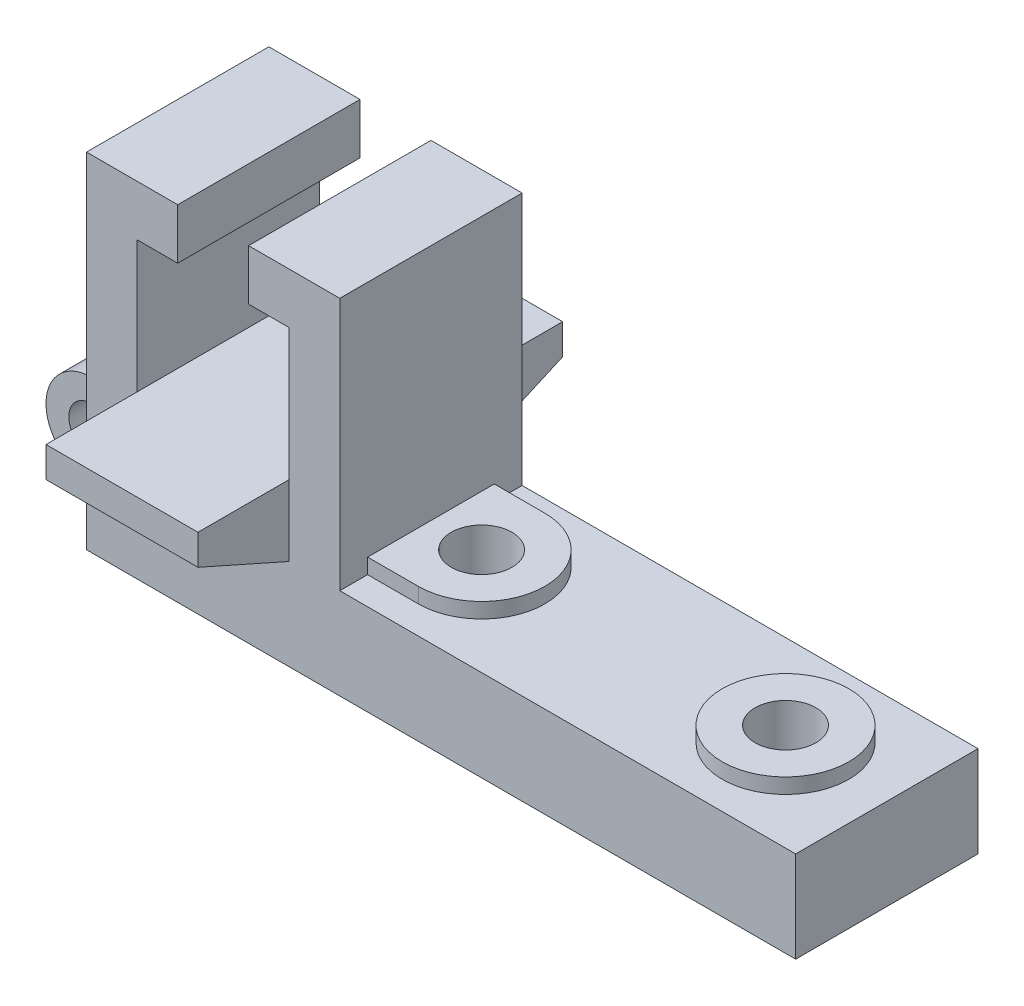
ISO-10303-21;
HEADER;
FILE_DESCRIPTION(('STEP AP214'),'2;1');
FILE_NAME('part.step','',(''),(''),'','','');
FILE_SCHEMA(('AUTOMOTIVE_DESIGN { 1 0 10303 214 1 1 1 1 }'));
ENDSEC;
DATA;
#1=APPLICATION_CONTEXT('core data for automotive mechanical design processes');
#2=APPLICATION_PROTOCOL_DEFINITION('international standard','automotive_design',2000,#1);
#3=PRODUCT_CONTEXT('',#1,'mechanical');
#4=PRODUCT('Part','Part','',(#3));
#5=PRODUCT_RELATED_PRODUCT_CATEGORY('part','',(#4));
#6=PRODUCT_DEFINITION_FORMATION('','',#4);
#7=PRODUCT_DEFINITION_CONTEXT('part definition',#1,'design');
#8=PRODUCT_DEFINITION('design','',#6,#7);
#9=PRODUCT_DEFINITION_SHAPE('','',#8);
#10=(LENGTH_UNIT() NAMED_UNIT(*) SI_UNIT(.MILLI.,.METRE.));
#11=(NAMED_UNIT(*) PLANE_ANGLE_UNIT() SI_UNIT($,.RADIAN.));
#12=(NAMED_UNIT(*) SI_UNIT($,.STERADIAN.) SOLID_ANGLE_UNIT());
#13=UNCERTAINTY_MEASURE_WITH_UNIT(LENGTH_MEASURE(1.E-05),#10,'distance_accuracy_value','');
#14=(GEOMETRIC_REPRESENTATION_CONTEXT(3) GLOBAL_UNCERTAINTY_ASSIGNED_CONTEXT((#13)) GLOBAL_UNIT_ASSIGNED_CONTEXT((#10,
#11,#12)) REPRESENTATION_CONTEXT('',''));
#15=CARTESIAN_POINT('',(0.,0.,0.));
#16=DIRECTION('',(0.,0.,1.));
#17=DIRECTION('',(1.,0.,0.));
#18=AXIS2_PLACEMENT_3D('',#15,#16,#17);
#19=CARTESIAN_POINT('',(140.,18.,36.));
#20=DIRECTION('',(0.,-1.,0.));
#21=DIRECTION('',(0.,0.,-1.));
#22=AXIS2_PLACEMENT_3D('',#19,#20,#21);
#23=PLANE('',#22);
#24=CARTESIAN_POINT('',(120.,18.,18.));
#25=DIRECTION('',(0.,-1.,0.));
#26=DIRECTION('',(0.,0.,-1.));
#27=AXIS2_PLACEMENT_3D('',#24,#25,#26);
#28=CIRCLE('',#27,12.5);
#29=CARTESIAN_POINT('',(120.,18.,5.50000000000001));
#30=VERTEX_POINT('',#29);
#31=EDGE_CURVE('E11',#30,#30,#28,.F.);
#32=ORIENTED_EDGE('',*,*,#31,.F.);
#33=EDGE_LOOP('',(#32));
#34=FACE_BOUND('',#33,.T.);
#35=DIRECTION('',(-1.,0.,0.));
#36=VECTOR('',#35,1.);
#37=CARTESIAN_POINT('',(60.,18.,5.49999999999999));
#38=LINE('',#37,#36);
#39=CARTESIAN_POINT('',(60.,18.,5.49999999999999));
#40=VERTEX_POINT('',#39);
#41=CARTESIAN_POINT('',(50.,18.,5.5));
#42=VERTEX_POINT('',#41);
#43=EDGE_CURVE('E58',#40,#42,#38,.T.);
#44=ORIENTED_EDGE('',*,*,#43,.F.);
#45=CARTESIAN_POINT('',(60.,18.,18.));
#46=DIRECTION('',(0.,1.,0.));
#47=DIRECTION('',(0.,0.,1.));
#48=AXIS2_PLACEMENT_3D('',#45,#46,#47);
#49=CIRCLE('',#48,12.5);
#50=CARTESIAN_POINT('',(60.,18.,30.5));
#51=VERTEX_POINT('',#50);
#52=EDGE_CURVE('E64',#51,#40,#49,.T.);
#53=ORIENTED_EDGE('',*,*,#52,.F.);
#54=DIRECTION('',(1.,0.,0.));
#55=VECTOR('',#54,1.);
#56=CARTESIAN_POINT('',(50.,18.,30.5));
#57=LINE('',#56,#55);
#58=CARTESIAN_POINT('',(50.,18.,30.5));
#59=VERTEX_POINT('',#58);
#60=EDGE_CURVE('E247',#59,#51,#57,.T.);
#61=ORIENTED_EDGE('',*,*,#60,.F.);
#62=DIRECTION('',(0.,0.,-1.));
#63=VECTOR('',#62,1.);
#64=CARTESIAN_POINT('',(50.,18.,36.));
#65=LINE('',#64,#63);
#66=CARTESIAN_POINT('',(50.,18.,36.));
#67=VERTEX_POINT('',#66);
#68=EDGE_CURVE('E323',#67,#59,#65,.T.);
#69=ORIENTED_EDGE('',*,*,#68,.F.);
#70=DIRECTION('',(-1.,0.,0.));
#71=VECTOR('',#70,1.);
#72=CARTESIAN_POINT('',(140.,18.,36.));
#73=LINE('',#72,#71);
#74=CARTESIAN_POINT('',(140.,18.,36.));
#75=VERTEX_POINT('',#74);
#76=EDGE_CURVE('E421',#75,#67,#73,.T.);
#77=ORIENTED_EDGE('',*,*,#76,.F.);
#78=DIRECTION('',(0.,0.,-1.));
#79=VECTOR('',#78,1.);
#80=CARTESIAN_POINT('',(140.,18.,36.));
#81=LINE('',#80,#79);
#82=CARTESIAN_POINT('',(140.,18.,0.));
#83=VERTEX_POINT('',#82);
#84=EDGE_CURVE('E428',#75,#83,#81,.T.);
#85=ORIENTED_EDGE('',*,*,#84,.T.);
#86=DIRECTION('',(-1.,0.,0.));
#87=VECTOR('',#86,1.);
#88=CARTESIAN_POINT('',(140.,18.,0.));
#89=LINE('',#88,#87);
#90=CARTESIAN_POINT('',(50.,18.,0.));
#91=VERTEX_POINT('',#90);
#92=EDGE_CURVE('E418',#83,#91,#89,.T.);
#93=ORIENTED_EDGE('',*,*,#92,.T.);
#94=EDGE_CURVE('E328',#42,#91,#65,.T.);
#95=ORIENTED_EDGE('',*,*,#94,.F.);
#96=EDGE_LOOP('',(#44,#53,#61,#69,#77,#85,#93,#95));
#97=FACE_BOUND('',#96,.T.);
#98=ADVANCED_FACE('F44',(#34,#97),#23,.F.);
#99=CARTESIAN_POINT('',(50.,18.,36.));
#100=DIRECTION('',(1.,0.,0.));
#101=DIRECTION('',(0.,0.,-1.));
#102=AXIS2_PLACEMENT_3D('',#99,#100,#101);
#103=PLANE('',#102);
#104=DIRECTION('',(0.,0.,1.));
#105=VECTOR('',#104,1.);
#106=CARTESIAN_POINT('',(50.,21.,5.49999999999999));
#107=LINE('',#106,#105);
#108=CARTESIAN_POINT('',(50.,21.,5.5));
#109=VERTEX_POINT('',#108);
#110=CARTESIAN_POINT('',(50.,21.,30.5));
#111=VERTEX_POINT('',#110);
#112=EDGE_CURVE('E238',#109,#111,#107,.T.);
#113=ORIENTED_EDGE('',*,*,#112,.F.);
#114=DIRECTION('',(0.,-1.,0.));
#115=VECTOR('',#114,1.);
#116=CARTESIAN_POINT('',(50.,21.,5.49999999999999));
#117=LINE('',#116,#115);
#118=EDGE_CURVE('E232',#109,#42,#117,.T.);
#119=ORIENTED_EDGE('',*,*,#118,.T.);
#120=ORIENTED_EDGE('',*,*,#94,.T.);
#121=DIRECTION('',(0.,-1.,0.));
#122=VECTOR('',#121,1.);
#123=CARTESIAN_POINT('',(50.,18.,0.));
#124=LINE('',#123,#122);
#125=CARTESIAN_POINT('',(50.,68.,0.));
#126=VERTEX_POINT('',#125);
#127=EDGE_CURVE('E321',#126,#91,#124,.T.);
#128=ORIENTED_EDGE('',*,*,#127,.F.);
#129=DIRECTION('',(0.,0.,-1.));
#130=VECTOR('',#129,1.);
#131=CARTESIAN_POINT('',(50.,68.,36.));
#132=LINE('',#131,#130);
#133=CARTESIAN_POINT('',(50.,68.,36.));
#134=VERTEX_POINT('',#133);
#135=EDGE_CURVE('E327',#134,#126,#132,.T.);
#136=ORIENTED_EDGE('',*,*,#135,.F.);
#137=DIRECTION('',(0.,-1.,0.));
#138=VECTOR('',#137,1.);
#139=CARTESIAN_POINT('',(50.,18.,36.));
#140=LINE('',#139,#138);
#141=EDGE_CURVE('E304',#134,#67,#140,.T.);
#142=ORIENTED_EDGE('',*,*,#141,.T.);
#143=ORIENTED_EDGE('',*,*,#68,.T.);
#144=DIRECTION('',(0.,-1.,0.));
#145=VECTOR('',#144,1.);
#146=CARTESIAN_POINT('',(50.,21.,30.5));
#147=LINE('',#146,#145);
#148=EDGE_CURVE('E256',#111,#59,#147,.T.);
#149=ORIENTED_EDGE('',*,*,#148,.F.);
#150=EDGE_LOOP('',(#113,#119,#120,#128,#136,#142,#143,#149));
#151=FACE_BOUND('',#150,.T.);
#152=ADVANCED_FACE('F523',(#151),#103,.T.);
#153=CARTESIAN_POINT('',(0.,18.,30.));
#154=DIRECTION('',(0.,1.,0.));
#155=DIRECTION('',(0.,0.,1.));
#156=AXIS2_PLACEMENT_3D('',#153,#154,#155);
#157=PLANE('',#156);
#158=DIRECTION('',(0.,0.,-1.));
#159=VECTOR('',#158,1.);
#160=CARTESIAN_POINT('',(-11.,18.,30.));
#161=LINE('',#160,#159);
#162=CARTESIAN_POINT('',(-11.,18.,24.));
#163=VERTEX_POINT('',#162);
#164=CARTESIAN_POINT('',(-11.,18.,12.));
#165=VERTEX_POINT('',#164);
#166=EDGE_CURVE('E287',#163,#165,#161,.T.);
#167=ORIENTED_EDGE('',*,*,#166,.F.);
#168=DIRECTION('',(-1.,0.,0.));
#169=VECTOR('',#168,1.);
#170=CARTESIAN_POINT('',(0.,18.,24.));
#171=LINE('',#170,#169);
#172=CARTESIAN_POINT('',(0.,18.,24.));
#173=VERTEX_POINT('',#172);
#174=EDGE_CURVE('E262',#173,#163,#171,.T.);
#175=ORIENTED_EDGE('',*,*,#174,.F.);
#176=DIRECTION('',(0.,0.,-1.));
#177=VECTOR('',#176,1.);
#178=CARTESIAN_POINT('',(0.,18.,30.));
#179=LINE('',#178,#177);
#180=CARTESIAN_POINT('',(0.,18.,12.));
#181=VERTEX_POINT('',#180);
#182=EDGE_CURVE('E286',#173,#181,#179,.T.);
#183=ORIENTED_EDGE('',*,*,#182,.T.);
#184=DIRECTION('',(1.,0.,0.));
#185=VECTOR('',#184,1.);
#186=CARTESIAN_POINT('',(0.,18.,12.));
#187=LINE('',#186,#185);
#188=EDGE_CURVE('E279',#165,#181,#187,.T.);
#189=ORIENTED_EDGE('',*,*,#188,.F.);
#190=EDGE_LOOP('',(#167,#175,#183,#189));
#191=FACE_BOUND('',#190,.T.);
#192=ADVANCED_FACE('F532',(#191),#157,.T.);
#193=CARTESIAN_POINT('',(-11.,9.,30.));
#194=DIRECTION('',(0.,0.,-1.));
#195=DIRECTION('',(-1.,0.,0.));
#196=AXIS2_PLACEMENT_3D('',#193,#194,#195);
#197=CYLINDRICAL_SURFACE('',#196,9.);
#198=DIRECTION('',(0.,0.,-1.));
#199=VECTOR('',#198,1.);
#200=CARTESIAN_POINT('',(-11.,0.,30.));
#201=LINE('',#200,#199);
#202=CARTESIAN_POINT('',(-10.9999999999999,0.,24.));
#203=VERTEX_POINT('',#202);
#204=CARTESIAN_POINT('',(-11.,0.,12.));
#205=VERTEX_POINT('',#204);
#206=EDGE_CURVE('E289',#203,#205,#201,.T.);
#207=ORIENTED_EDGE('',*,*,#206,.F.);
#208=CARTESIAN_POINT('',(-11.,9.,24.));
#209=DIRECTION('',(0.,0.,1.));
#210=DIRECTION('',(1.,0.,0.));
#211=AXIS2_PLACEMENT_3D('',#208,#209,#210);
#212=CIRCLE('',#211,9.);
#213=EDGE_CURVE('E269',#163,#203,#212,.T.);
#214=ORIENTED_EDGE('',*,*,#213,.F.);
#215=ORIENTED_EDGE('',*,*,#166,.T.);
#216=CARTESIAN_POINT('',(-11.,9.,12.));
#217=DIRECTION('',(0.,0.,-1.));
#218=DIRECTION('',(-1.,0.,0.));
#219=AXIS2_PLACEMENT_3D('',#216,#217,#218);
#220=CIRCLE('',#219,9.);
#221=EDGE_CURVE('E280',#205,#165,#220,.T.);
#222=ORIENTED_EDGE('',*,*,#221,.F.);
#223=EDGE_LOOP('',(#207,#214,#215,#222));
#224=FACE_BOUND('',#223,.T.);
#225=ADVANCED_FACE('F571',(#224),#197,.T.);
#226=CARTESIAN_POINT('',(0.,18.,36.));
#227=DIRECTION('',(1.,0.,0.));
#228=DIRECTION('',(0.,0.,-1.));
#229=AXIS2_PLACEMENT_3D('',#226,#227,#228);
#230=PLANE('',#229);
#231=ORIENTED_EDGE('',*,*,#182,.F.);
#232=DIRECTION('',(0.,1.,0.));
#233=VECTOR('',#232,1.);
#234=CARTESIAN_POINT('',(0.,0.,24.));
#235=LINE('',#234,#233);
#236=CARTESIAN_POINT('',(0.,0.,24.));
#237=VERTEX_POINT('',#236);
#238=EDGE_CURVE('E261',#237,#173,#235,.T.);
#239=ORIENTED_EDGE('',*,*,#238,.F.);
#240=DIRECTION('',(0.,0.,-1.));
#241=VECTOR('',#240,1.);
#242=CARTESIAN_POINT('',(0.,0.,36.));
#243=LINE('',#242,#241);
#244=CARTESIAN_POINT('',(0.,0.,36.));
#245=VERTEX_POINT('',#244);
#246=EDGE_CURVE('E437',#245,#237,#243,.T.);
#247=ORIENTED_EDGE('',*,*,#246,.F.);
#248=DIRECTION('',(0.,-1.,0.));
#249=VECTOR('',#248,1.);
#250=CARTESIAN_POINT('',(0.,18.,36.));
#251=LINE('',#250,#249);
#252=CARTESIAN_POINT('',(0.,68.,36.));
#253=VERTEX_POINT('',#252);
#254=EDGE_CURVE('E414',#253,#245,#251,.T.);
#255=ORIENTED_EDGE('',*,*,#254,.F.);
#256=DIRECTION('',(0.,0.,1.));
#257=VECTOR('',#256,1.);
#258=CARTESIAN_POINT('',(0.,68.,0.));
#259=LINE('',#258,#257);
#260=CARTESIAN_POINT('',(0.,68.,0.));
#261=VERTEX_POINT('',#260);
#262=EDGE_CURVE('E403',#261,#253,#259,.T.);
#263=ORIENTED_EDGE('',*,*,#262,.F.);
#264=DIRECTION('',(0.,-1.,0.));
#265=VECTOR('',#264,1.);
#266=CARTESIAN_POINT('',(0.,18.,0.));
#267=LINE('',#266,#265);
#268=CARTESIAN_POINT('',(0.,0.,0.));
#269=VERTEX_POINT('',#268);
#270=EDGE_CURVE('E407',#261,#269,#267,.T.);
#271=ORIENTED_EDGE('',*,*,#270,.T.);
#272=DIRECTION('',(0.,0.,-1.));
#273=VECTOR('',#272,1.);
#274=CARTESIAN_POINT('',(0.,0.,12.));
#275=LINE('',#274,#273);
#276=CARTESIAN_POINT('',(0.,0.,12.));
#277=VERTEX_POINT('',#276);
#278=EDGE_CURVE('E283',#277,#269,#275,.T.);
#279=ORIENTED_EDGE('',*,*,#278,.F.);
#280=DIRECTION('',(0.,-1.,0.));
#281=VECTOR('',#280,1.);
#282=CARTESIAN_POINT('',(0.,0.,12.));
#283=LINE('',#282,#281);
#284=EDGE_CURVE('E272',#181,#277,#283,.T.);
#285=ORIENTED_EDGE('',*,*,#284,.F.);
#286=EDGE_LOOP('',(#231,#239,#247,#255,#263,#271,#279,#285));
#287=FACE_BOUND('',#286,.T.);
#288=ADVANCED_FACE('F50',(#287),#230,.F.);
#289=CARTESIAN_POINT('',(40.,0.,0.));
#290=DIRECTION('',(-1.,0.,0.));
#291=DIRECTION('',(0.,0.,1.));
#292=AXIS2_PLACEMENT_3D('',#289,#290,#291);
#293=PLANE('',#292);
#294=DIRECTION('',(0.,1.,0.));
#295=VECTOR('',#294,1.);
#296=CARTESIAN_POINT('',(40.,18.,0.));
#297=LINE('',#296,#295);
#298=CARTESIAN_POINT('',(40.,18.,0.));
#299=VERTEX_POINT('',#298);
#300=CARTESIAN_POINT('',(40.,32.,0.));
#301=VERTEX_POINT('',#300);
#302=EDGE_CURVE('E307',#299,#301,#297,.T.);
#303=ORIENTED_EDGE('',*,*,#302,.F.);
#304=DIRECTION('',(0.,0.406138466053448,-0.913811548620257));
#305=VECTOR('',#304,1.);
#306=CARTESIAN_POINT('',(40.,26.,-18.));
#307=LINE('',#306,#305);
#308=CARTESIAN_POINT('',(40.,26.,-18.));
#309=VERTEX_POINT('',#308);
#310=EDGE_CURVE('E340',#299,#309,#307,.T.);
#311=ORIENTED_EDGE('',*,*,#310,.T.);
#312=DIRECTION('',(0.,1.,0.));
#313=VECTOR('',#312,1.);
#314=CARTESIAN_POINT('',(40.,32.,-18.));
#315=LINE('',#314,#313);
#316=CARTESIAN_POINT('',(40.,32.,-18.));
#317=VERTEX_POINT('',#316);
#318=EDGE_CURVE('E339',#309,#317,#315,.T.);
#319=ORIENTED_EDGE('',*,*,#318,.T.);
#320=DIRECTION('',(0.,0.,1.));
#321=VECTOR('',#320,1.);
#322=CARTESIAN_POINT('',(40.,32.,18.));
#323=LINE('',#322,#321);
#324=EDGE_CURVE('E342',#317,#301,#323,.T.);
#325=ORIENTED_EDGE('',*,*,#324,.T.);
#326=EDGE_LOOP('',(#303,#311,#319,#325));
#327=FACE_BOUND('',#326,.T.);
#328=ADVANCED_FACE('F496',(#327),#293,.F.);
#329=CARTESIAN_POINT('',(10.,18.,0.));
#330=DIRECTION('',(1.,0.,0.));
#331=DIRECTION('',(0.,0.,-1.));
#332=AXIS2_PLACEMENT_3D('',#329,#330,#331);
#333=PLANE('',#332);
#334=DIRECTION('',(0.,1.,0.));
#335=VECTOR('',#334,1.);
#336=CARTESIAN_POINT('',(10.,18.,36.));
#337=LINE('',#336,#335);
#338=CARTESIAN_POINT('',(10.,32.,36.));
#339=VERTEX_POINT('',#338);
#340=CARTESIAN_POINT('',(10.,58.,36.));
#341=VERTEX_POINT('',#340);
#342=EDGE_CURVE('E377',#339,#341,#337,.T.);
#343=ORIENTED_EDGE('',*,*,#342,.F.);
#344=DIRECTION('',(0.,0.,-1.));
#345=VECTOR('',#344,1.);
#346=CARTESIAN_POINT('',(10.,32.,0.));
#347=LINE('',#346,#345);
#348=CARTESIAN_POINT('',(10.,32.,0.));
#349=VERTEX_POINT('',#348);
#350=EDGE_CURVE('E52',#339,#349,#347,.T.);
#351=ORIENTED_EDGE('',*,*,#350,.T.);
#352=DIRECTION('',(0.,1.,0.));
#353=VECTOR('',#352,1.);
#354=CARTESIAN_POINT('',(10.,18.,0.));
#355=LINE('',#354,#353);
#356=CARTESIAN_POINT('',(10.,58.,0.));
#357=VERTEX_POINT('',#356);
#358=EDGE_CURVE('E384',#349,#357,#355,.T.);
#359=ORIENTED_EDGE('',*,*,#358,.T.);
#360=DIRECTION('',(0.,0.,1.));
#361=VECTOR('',#360,1.);
#362=CARTESIAN_POINT('',(10.,58.,0.));
#363=LINE('',#362,#361);
#364=EDGE_CURVE('E395',#357,#341,#363,.T.);
#365=ORIENTED_EDGE('',*,*,#364,.T.);
#366=EDGE_LOOP('',(#343,#351,#359,#365));
#367=FACE_BOUND('',#366,.T.);
#368=ADVANCED_FACE('F444',(#367),#333,.T.);
#369=CARTESIAN_POINT('',(0.,0.,36.));
#370=DIRECTION('',(0.,1.,0.));
#371=DIRECTION('',(0.,0.,1.));
#372=AXIS2_PLACEMENT_3D('',#369,#370,#371);
#373=PLANE('',#372);
#374=CARTESIAN_POINT('',(120.,0.,18.));
#375=DIRECTION('',(0.,1.,0.));
#376=DIRECTION('',(0.,0.,1.));
#377=AXIS2_PLACEMENT_3D('',#374,#375,#376);
#378=CIRCLE('',#377,6.);
#379=CARTESIAN_POINT('',(120.,0.,24.));
#380=VERTEX_POINT('',#379);
#381=EDGE_CURVE('E552',#380,#380,#378,.T.);
#382=ORIENTED_EDGE('',*,*,#381,.T.);
#383=EDGE_LOOP('',(#382));
#384=FACE_BOUND('',#383,.T.);
#385=CARTESIAN_POINT('',(60.,0.,18.));
#386=DIRECTION('',(0.,1.,0.));
#387=DIRECTION('',(0.,0.,1.));
#388=AXIS2_PLACEMENT_3D('',#385,#386,#387);
#389=CIRCLE('',#388,6.);
#390=CARTESIAN_POINT('',(60.,0.,24.));
#391=VERTEX_POINT('',#390);
#392=EDGE_CURVE('E558',#391,#391,#389,.T.);
#393=ORIENTED_EDGE('',*,*,#392,.T.);
#394=EDGE_LOOP('',(#393));
#395=FACE_BOUND('',#394,.T.);
#396=ORIENTED_EDGE('',*,*,#246,.T.);
#397=DIRECTION('',(1.,0.,0.));
#398=VECTOR('',#397,1.);
#399=CARTESIAN_POINT('',(-10.9999999999999,0.,24.));
#400=LINE('',#399,#398);
#401=EDGE_CURVE('E270',#203,#237,#400,.T.);
#402=ORIENTED_EDGE('',*,*,#401,.F.);
#403=ORIENTED_EDGE('',*,*,#206,.T.);
#404=DIRECTION('',(-1.,0.,0.));
#405=VECTOR('',#404,1.);
#406=CARTESIAN_POINT('',(-11.,0.,12.));
#407=LINE('',#406,#405);
#408=EDGE_CURVE('E274',#277,#205,#407,.T.);
#409=ORIENTED_EDGE('',*,*,#408,.F.);
#410=ORIENTED_EDGE('',*,*,#278,.T.);
#411=DIRECTION('',(1.,0.,0.));
#412=VECTOR('',#411,1.);
#413=CARTESIAN_POINT('',(0.,0.,0.));
#414=LINE('',#413,#412);
#415=CARTESIAN_POINT('',(140.,0.,0.));
#416=VERTEX_POINT('',#415);
#417=EDGE_CURVE('E426',#269,#416,#414,.T.);
#418=ORIENTED_EDGE('',*,*,#417,.T.);
#419=DIRECTION('',(0.,0.,-1.));
#420=VECTOR('',#419,1.);
#421=CARTESIAN_POINT('',(140.,0.,36.));
#422=LINE('',#421,#420);
#423=CARTESIAN_POINT('',(140.,0.,36.));
#424=VERTEX_POINT('',#423);
#425=EDGE_CURVE('E436',#424,#416,#422,.T.);
#426=ORIENTED_EDGE('',*,*,#425,.F.);
#427=DIRECTION('',(1.,0.,0.));
#428=VECTOR('',#427,1.);
#429=CARTESIAN_POINT('',(0.,0.,36.));
#430=LINE('',#429,#428);
#431=EDGE_CURVE('E420',#245,#424,#430,.T.);
#432=ORIENTED_EDGE('',*,*,#431,.F.);
#433=EDGE_LOOP('',(#396,#402,#403,#409,#410,#418,#426,#432));
#434=FACE_BOUND('',#433,.T.);
#435=ADVANCED_FACE('F539',(#384,#395,#434),#373,.F.);
#436=CARTESIAN_POINT('',(140.,0.,36.));
#437=DIRECTION('',(-1.,0.,0.));
#438=DIRECTION('',(0.,0.,1.));
#439=AXIS2_PLACEMENT_3D('',#436,#437,#438);
#440=PLANE('',#439);
#441=DIRECTION('',(0.,1.,0.));
#442=VECTOR('',#441,1.);
#443=CARTESIAN_POINT('',(140.,0.,0.));
#444=LINE('',#443,#442);
#445=EDGE_CURVE('E427',#416,#83,#444,.T.);
#446=ORIENTED_EDGE('',*,*,#445,.T.);
#447=ORIENTED_EDGE('',*,*,#84,.F.);
#448=DIRECTION('',(0.,1.,0.));
#449=VECTOR('',#448,1.);
#450=CARTESIAN_POINT('',(140.,0.,36.));
#451=LINE('',#450,#449);
#452=EDGE_CURVE('E423',#424,#75,#451,.T.);
#453=ORIENTED_EDGE('',*,*,#452,.F.);
#454=ORIENTED_EDGE('',*,*,#425,.T.);
#455=EDGE_LOOP('',(#446,#447,#453,#454));
#456=FACE_BOUND('',#455,.T.);
#457=ADVANCED_FACE('F537',(#456),#440,.F.);
#458=CARTESIAN_POINT('',(0.,0.,36.));
#459=DIRECTION('',(0.,0.,1.));
#460=DIRECTION('',(1.,0.,0.));
#461=AXIS2_PLACEMENT_3D('',#458,#459,#460);
#462=PLANE('',#461);
#463=ORIENTED_EDGE('',*,*,#254,.T.);
#464=ORIENTED_EDGE('',*,*,#431,.T.);
#465=ORIENTED_EDGE('',*,*,#452,.T.);
#466=ORIENTED_EDGE('',*,*,#76,.T.);
#467=ORIENTED_EDGE('',*,*,#141,.F.);
#468=DIRECTION('',(1.,0.,0.));
#469=VECTOR('',#468,1.);
#470=CARTESIAN_POINT('',(50.,68.,36.));
#471=LINE('',#470,#469);
#472=CARTESIAN_POINT('',(32.,68.,36.));
#473=VERTEX_POINT('',#472);
#474=EDGE_CURVE('E305',#473,#134,#471,.T.);
#475=ORIENTED_EDGE('',*,*,#474,.F.);
#476=DIRECTION('',(0.,1.,0.));
#477=VECTOR('',#476,1.);
#478=CARTESIAN_POINT('',(32.,68.,36.));
#479=LINE('',#478,#477);
#480=CARTESIAN_POINT('',(32.,58.,36.));
#481=VERTEX_POINT('',#480);
#482=EDGE_CURVE('E299',#481,#473,#479,.T.);
#483=ORIENTED_EDGE('',*,*,#482,.F.);
#484=DIRECTION('',(-1.,0.,0.));
#485=VECTOR('',#484,1.);
#486=CARTESIAN_POINT('',(40.,58.,36.));
#487=LINE('',#486,#485);
#488=CARTESIAN_POINT('',(40.,58.,36.));
#489=VERTEX_POINT('',#488);
#490=EDGE_CURVE('E294',#489,#481,#487,.T.);
#491=ORIENTED_EDGE('',*,*,#490,.F.);
#492=DIRECTION('',(0.,1.,0.));
#493=VECTOR('',#492,1.);
#494=CARTESIAN_POINT('',(40.,18.,36.));
#495=LINE('',#494,#493);
#496=CARTESIAN_POINT('',(40.,32.,36.));
#497=VERTEX_POINT('',#496);
#498=EDGE_CURVE('E298',#497,#489,#495,.T.);
#499=ORIENTED_EDGE('',*,*,#498,.F.);
#500=CARTESIAN_POINT('',(40.,18.,36.));
#501=VERTEX_POINT('',#500);
#502=EDGE_CURVE('E291',#501,#497,#495,.T.);
#503=ORIENTED_EDGE('',*,*,#502,.F.);
#504=DIRECTION('',(-1.,0.,0.));
#505=VECTOR('',#504,1.);
#506=CARTESIAN_POINT('',(40.,18.,36.));
#507=LINE('',#506,#505);
#508=CARTESIAN_POINT('',(10.,18.,36.));
#509=VERTEX_POINT('',#508);
#510=EDGE_CURVE('E349',#501,#509,#507,.T.);
#511=ORIENTED_EDGE('',*,*,#510,.T.);
#512=EDGE_CURVE('E393',#509,#339,#337,.T.);
#513=ORIENTED_EDGE('',*,*,#512,.T.);
#514=ORIENTED_EDGE('',*,*,#342,.T.);
#515=DIRECTION('',(1.,0.,0.));
#516=VECTOR('',#515,1.);
#517=CARTESIAN_POINT('',(10.,58.,36.));
#518=LINE('',#517,#516);
#519=CARTESIAN_POINT('',(18.,58.,36.));
#520=VERTEX_POINT('',#519);
#521=EDGE_CURVE('E399',#341,#520,#518,.T.);
#522=ORIENTED_EDGE('',*,*,#521,.T.);
#523=DIRECTION('',(0.,1.,0.));
#524=VECTOR('',#523,1.);
#525=CARTESIAN_POINT('',(18.,68.,36.));
#526=LINE('',#525,#524);
#527=CARTESIAN_POINT('',(18.,68.,36.));
#528=VERTEX_POINT('',#527);
#529=EDGE_CURVE('E398',#520,#528,#526,.T.);
#530=ORIENTED_EDGE('',*,*,#529,.T.);
#531=DIRECTION('',(-1.,0.,0.));
#532=VECTOR('',#531,1.);
#533=CARTESIAN_POINT('',(0.,68.,36.));
#534=LINE('',#533,#532);
#535=EDGE_CURVE('E405',#528,#253,#534,.T.);
#536=ORIENTED_EDGE('',*,*,#535,.T.);
#537=EDGE_LOOP('',(#463,#464,#465,#466,#467,#475,#483,#491,#499,#503,#511,#513,#514,#522,#530,#536));
#538=FACE_BOUND('',#537,.T.);
#539=ADVANCED_FACE('F464',(#538),#462,.T.);
#540=CARTESIAN_POINT('',(0.,0.,0.));
#541=DIRECTION('',(0.,0.,1.));
#542=DIRECTION('',(1.,0.,0.));
#543=AXIS2_PLACEMENT_3D('',#540,#541,#542);
#544=PLANE('',#543);
#545=ORIENTED_EDGE('',*,*,#417,.F.);
#546=ORIENTED_EDGE('',*,*,#270,.F.);
#547=DIRECTION('',(-1.,0.,0.));
#548=VECTOR('',#547,1.);
#549=CARTESIAN_POINT('',(0.,68.,0.));
#550=LINE('',#549,#548);
#551=CARTESIAN_POINT('',(18.,68.,0.));
#552=VERTEX_POINT('',#551);
#553=EDGE_CURVE('E388',#552,#261,#550,.T.);
#554=ORIENTED_EDGE('',*,*,#553,.F.);
#555=DIRECTION('',(0.,1.,0.));
#556=VECTOR('',#555,1.);
#557=CARTESIAN_POINT('',(18.,68.,0.));
#558=LINE('',#557,#556);
#559=CARTESIAN_POINT('',(18.,58.,0.));
#560=VERTEX_POINT('',#559);
#561=EDGE_CURVE('E386',#560,#552,#558,.T.);
#562=ORIENTED_EDGE('',*,*,#561,.F.);
#563=DIRECTION('',(1.,0.,0.));
#564=VECTOR('',#563,1.);
#565=CARTESIAN_POINT('',(10.,58.,0.));
#566=LINE('',#565,#564);
#567=EDGE_CURVE('E385',#357,#560,#566,.T.);
#568=ORIENTED_EDGE('',*,*,#567,.F.);
#569=ORIENTED_EDGE('',*,*,#358,.F.);
#570=CARTESIAN_POINT('',(10.,18.,0.));
#571=VERTEX_POINT('',#570);
#572=EDGE_CURVE('E378',#571,#349,#355,.T.);
#573=ORIENTED_EDGE('',*,*,#572,.F.);
#574=DIRECTION('',(-1.,0.,0.));
#575=VECTOR('',#574,1.);
#576=CARTESIAN_POINT('',(40.,18.,0.));
#577=LINE('',#576,#575);
#578=EDGE_CURVE('E376',#299,#571,#577,.T.);
#579=ORIENTED_EDGE('',*,*,#578,.F.);
#580=ORIENTED_EDGE('',*,*,#302,.T.);
#581=CARTESIAN_POINT('',(40.,58.,0.));
#582=VERTEX_POINT('',#581);
#583=EDGE_CURVE('E288',#301,#582,#297,.T.);
#584=ORIENTED_EDGE('',*,*,#583,.T.);
#585=DIRECTION('',(-1.,0.,0.));
#586=VECTOR('',#585,1.);
#587=CARTESIAN_POINT('',(40.,58.,0.));
#588=LINE('',#587,#586);
#589=CARTESIAN_POINT('',(32.,58.,0.));
#590=VERTEX_POINT('',#589);
#591=EDGE_CURVE('E315',#582,#590,#588,.T.);
#592=ORIENTED_EDGE('',*,*,#591,.T.);
#593=DIRECTION('',(0.,1.,0.));
#594=VECTOR('',#593,1.);
#595=CARTESIAN_POINT('',(32.,68.,0.));
#596=LINE('',#595,#594);
#597=CARTESIAN_POINT('',(32.,68.,0.));
#598=VERTEX_POINT('',#597);
#599=EDGE_CURVE('E314',#590,#598,#596,.T.);
#600=ORIENTED_EDGE('',*,*,#599,.T.);
#601=DIRECTION('',(1.,0.,0.));
#602=VECTOR('',#601,1.);
#603=CARTESIAN_POINT('',(50.,68.,0.));
#604=LINE('',#603,#602);
#605=EDGE_CURVE('E319',#598,#126,#604,.T.);
#606=ORIENTED_EDGE('',*,*,#605,.T.);
#607=ORIENTED_EDGE('',*,*,#127,.T.);
#608=ORIENTED_EDGE('',*,*,#92,.F.);
#609=ORIENTED_EDGE('',*,*,#445,.F.);
#610=EDGE_LOOP('',(#545,#546,#554,#562,#568,#569,#573,#579,#580,#584,#592,#600,#606,#607,#608,#609));
#611=FACE_BOUND('',#610,.T.);
#612=ADVANCED_FACE('F455',(#611),#544,.F.);
#613=CARTESIAN_POINT('',(0.,68.,0.));
#614=DIRECTION('',(0.,1.,0.));
#615=DIRECTION('',(0.,0.,1.));
#616=AXIS2_PLACEMENT_3D('',#613,#614,#615);
#617=PLANE('',#616);
#618=ORIENTED_EDGE('',*,*,#535,.F.);
#619=DIRECTION('',(0.,0.,1.));
#620=VECTOR('',#619,1.);
#621=CARTESIAN_POINT('',(18.,68.,0.));
#622=LINE('',#621,#620);
#623=EDGE_CURVE('E408',#552,#528,#622,.T.);
#624=ORIENTED_EDGE('',*,*,#623,.F.);
#625=ORIENTED_EDGE('',*,*,#553,.T.);
#626=ORIENTED_EDGE('',*,*,#262,.T.);
#627=EDGE_LOOP('',(#618,#624,#625,#626));
#628=FACE_BOUND('',#627,.T.);
#629=ADVANCED_FACE('F896',(#628),#617,.T.);
#630=CARTESIAN_POINT('',(18.,68.,0.));
#631=DIRECTION('',(1.,0.,0.));
#632=DIRECTION('',(0.,0.,-1.));
#633=AXIS2_PLACEMENT_3D('',#630,#631,#632);
#634=PLANE('',#633);
#635=ORIENTED_EDGE('',*,*,#529,.F.);
#636=DIRECTION('',(0.,0.,1.));
#637=VECTOR('',#636,1.);
#638=CARTESIAN_POINT('',(18.,58.,0.));
#639=LINE('',#638,#637);
#640=EDGE_CURVE('E411',#560,#520,#639,.T.);
#641=ORIENTED_EDGE('',*,*,#640,.F.);
#642=ORIENTED_EDGE('',*,*,#561,.T.);
#643=ORIENTED_EDGE('',*,*,#623,.T.);
#644=EDGE_LOOP('',(#635,#641,#642,#643));
#645=FACE_BOUND('',#644,.T.);
#646=ADVANCED_FACE('F516',(#645),#634,.T.);
#647=CARTESIAN_POINT('',(10.,58.,0.));
#648=DIRECTION('',(0.,-1.,0.));
#649=DIRECTION('',(0.,0.,-1.));
#650=AXIS2_PLACEMENT_3D('',#647,#648,#649);
#651=PLANE('',#650);
#652=ORIENTED_EDGE('',*,*,#521,.F.);
#653=ORIENTED_EDGE('',*,*,#364,.F.);
#654=ORIENTED_EDGE('',*,*,#567,.T.);
#655=ORIENTED_EDGE('',*,*,#640,.T.);
#656=EDGE_LOOP('',(#652,#653,#654,#655));
#657=FACE_BOUND('',#656,.T.);
#658=ADVANCED_FACE('F458',(#657),#651,.T.);
#659=CARTESIAN_POINT('',(10.,0.,0.));
#660=DIRECTION('',(-1.,0.,0.));
#661=DIRECTION('',(0.,0.,1.));
#662=AXIS2_PLACEMENT_3D('',#659,#660,#661);
#663=PLANE('',#662);
#664=ORIENTED_EDGE('',*,*,#572,.T.);
#665=DIRECTION('',(0.,0.,1.));
#666=VECTOR('',#665,1.);
#667=CARTESIAN_POINT('',(10.,32.,18.));
#668=LINE('',#667,#666);
#669=CARTESIAN_POINT('',(10.,32.,-18.));
#670=VERTEX_POINT('',#669);
#671=EDGE_CURVE('E358',#670,#349,#668,.T.);
#672=ORIENTED_EDGE('',*,*,#671,.F.);
#673=DIRECTION('',(0.,1.,0.));
#674=VECTOR('',#673,1.);
#675=CARTESIAN_POINT('',(10.,32.,-18.));
#676=LINE('',#675,#674);
#677=CARTESIAN_POINT('',(10.,26.,-18.));
#678=VERTEX_POINT('',#677);
#679=EDGE_CURVE('E351',#678,#670,#676,.T.);
#680=ORIENTED_EDGE('',*,*,#679,.F.);
#681=DIRECTION('',(0.,0.406138466053448,-0.913811548620257));
#682=VECTOR('',#681,1.);
#683=CARTESIAN_POINT('',(10.,26.,-18.));
#684=LINE('',#683,#682);
#685=EDGE_CURVE('E330',#571,#678,#684,.T.);
#686=ORIENTED_EDGE('',*,*,#685,.F.);
#687=EDGE_LOOP('',(#664,#672,#680,#686));
#688=FACE_BOUND('',#687,.T.);
#689=ADVANCED_FACE('F510',(#688),#663,.T.);
#690=CARTESIAN_POINT('',(40.,26.,-18.));
#691=DIRECTION('',(0.,0.913811548620257,0.406138466053448));
#692=DIRECTION('',(0.,-0.406138466053448,0.913811548620257));
#693=AXIS2_PLACEMENT_3D('',#690,#691,#692);
#694=PLANE('',#693);
#695=ORIENTED_EDGE('',*,*,#685,.T.);
#696=DIRECTION('',(-1.,0.,0.));
#697=VECTOR('',#696,1.);
#698=CARTESIAN_POINT('',(40.,26.,-18.));
#699=LINE('',#698,#697);
#700=EDGE_CURVE('E373',#309,#678,#699,.T.);
#701=ORIENTED_EDGE('',*,*,#700,.F.);
#702=ORIENTED_EDGE('',*,*,#310,.F.);
#703=ORIENTED_EDGE('',*,*,#578,.T.);
#704=EDGE_LOOP('',(#695,#701,#702,#703));
#705=FACE_BOUND('',#704,.T.);
#706=ADVANCED_FACE('F497',(#705),#694,.F.);
#707=CARTESIAN_POINT('',(40.,32.,-18.));
#708=DIRECTION('',(0.,0.,1.));
#709=DIRECTION('',(1.,0.,0.));
#710=AXIS2_PLACEMENT_3D('',#707,#708,#709);
#711=PLANE('',#710);
#712=ORIENTED_EDGE('',*,*,#679,.T.);
#713=DIRECTION('',(-1.,0.,0.));
#714=VECTOR('',#713,1.);
#715=CARTESIAN_POINT('',(40.,32.,-18.));
#716=LINE('',#715,#714);
#717=EDGE_CURVE('E369',#317,#670,#716,.T.);
#718=ORIENTED_EDGE('',*,*,#717,.F.);
#719=ORIENTED_EDGE('',*,*,#318,.F.);
#720=ORIENTED_EDGE('',*,*,#700,.T.);
#721=EDGE_LOOP('',(#712,#718,#719,#720));
#722=FACE_BOUND('',#721,.T.);
#723=ADVANCED_FACE('F504',(#722),#711,.F.);
#724=CARTESIAN_POINT('',(40.,32.,18.));
#725=DIRECTION('',(0.,-1.,0.));
#726=DIRECTION('',(0.,0.,-1.));
#727=AXIS2_PLACEMENT_3D('',#724,#725,#726);
#728=PLANE('',#727);
#729=ORIENTED_EDGE('',*,*,#671,.T.);
#730=ORIENTED_EDGE('',*,*,#350,.F.);
#731=CARTESIAN_POINT('',(10.,32.,54.));
#732=VERTEX_POINT('',#731);
#733=EDGE_CURVE('E352',#339,#732,#668,.T.);
#734=ORIENTED_EDGE('',*,*,#733,.T.);
#735=DIRECTION('',(-1.,0.,0.));
#736=VECTOR('',#735,1.);
#737=CARTESIAN_POINT('',(40.,32.,54.));
#738=LINE('',#737,#736);
#739=CARTESIAN_POINT('',(40.,32.,54.));
#740=VERTEX_POINT('',#739);
#741=EDGE_CURVE('E370',#740,#732,#738,.T.);
#742=ORIENTED_EDGE('',*,*,#741,.F.);
#743=EDGE_CURVE('E345',#497,#740,#323,.T.);
#744=ORIENTED_EDGE('',*,*,#743,.F.);
#745=EDGE_CURVE('E346',#301,#497,#323,.T.);
#746=ORIENTED_EDGE('',*,*,#745,.F.);
#747=ORIENTED_EDGE('',*,*,#324,.F.);
#748=ORIENTED_EDGE('',*,*,#717,.T.);
#749=EDGE_LOOP('',(#729,#730,#734,#742,#744,#746,#747,#748));
#750=FACE_BOUND('',#749,.T.);
#751=ADVANCED_FACE('F480',(#750),#728,.F.);
#752=CARTESIAN_POINT('',(40.,32.,54.));
#753=DIRECTION('',(0.,0.,-1.));
#754=DIRECTION('',(-1.,0.,0.));
#755=AXIS2_PLACEMENT_3D('',#752,#753,#754);
#756=PLANE('',#755);
#757=DIRECTION('',(0.,-1.,0.));
#758=VECTOR('',#757,1.);
#759=CARTESIAN_POINT('',(10.,32.,54.));
#760=LINE('',#759,#758);
#761=CARTESIAN_POINT('',(10.,26.,54.));
#762=VERTEX_POINT('',#761);
#763=EDGE_CURVE('E356',#732,#762,#760,.T.);
#764=ORIENTED_EDGE('',*,*,#763,.T.);
#765=DIRECTION('',(-1.,0.,0.));
#766=VECTOR('',#765,1.);
#767=CARTESIAN_POINT('',(40.,26.,54.));
#768=LINE('',#767,#766);
#769=CARTESIAN_POINT('',(40.,26.,54.));
#770=VERTEX_POINT('',#769);
#771=EDGE_CURVE('E364',#770,#762,#768,.T.);
#772=ORIENTED_EDGE('',*,*,#771,.F.);
#773=DIRECTION('',(0.,-1.,0.));
#774=VECTOR('',#773,1.);
#775=CARTESIAN_POINT('',(40.,32.,54.));
#776=LINE('',#775,#774);
#777=EDGE_CURVE('E344',#740,#770,#776,.T.);
#778=ORIENTED_EDGE('',*,*,#777,.F.);
#779=ORIENTED_EDGE('',*,*,#741,.T.);
#780=EDGE_LOOP('',(#764,#772,#778,#779));
#781=FACE_BOUND('',#780,.T.);
#782=ADVANCED_FACE('F473',(#781),#756,.F.);
#783=CARTESIAN_POINT('',(40.,26.,54.));
#784=DIRECTION('',(0.,0.913811548620257,-0.406138466053448));
#785=DIRECTION('',(0.,0.406138466053448,0.913811548620257));
#786=AXIS2_PLACEMENT_3D('',#783,#784,#785);
#787=PLANE('',#786);
#788=DIRECTION('',(0.,-0.406138466053448,-0.913811548620257));
#789=VECTOR('',#788,1.);
#790=CARTESIAN_POINT('',(10.,26.,54.));
#791=LINE('',#790,#789);
#792=EDGE_CURVE('E338',#762,#509,#791,.T.);
#793=ORIENTED_EDGE('',*,*,#792,.T.);
#794=ORIENTED_EDGE('',*,*,#510,.F.);
#795=DIRECTION('',(0.,-0.406138466053448,-0.913811548620257));
#796=VECTOR('',#795,1.);
#797=CARTESIAN_POINT('',(40.,26.,54.));
#798=LINE('',#797,#796);
#799=EDGE_CURVE('E348',#770,#501,#798,.T.);
#800=ORIENTED_EDGE('',*,*,#799,.F.);
#801=ORIENTED_EDGE('',*,*,#771,.T.);
#802=EDGE_LOOP('',(#793,#794,#800,#801));
#803=FACE_BOUND('',#802,.T.);
#804=ADVANCED_FACE('F469',(#803),#787,.F.);
#805=ORIENTED_EDGE('',*,*,#799,.T.);
#806=ORIENTED_EDGE('',*,*,#502,.T.);
#807=ORIENTED_EDGE('',*,*,#743,.T.);
#808=ORIENTED_EDGE('',*,*,#777,.T.);
#809=EDGE_LOOP('',(#805,#806,#807,#808));
#810=FACE_BOUND('',#809,.T.);
#811=ADVANCED_FACE('F521',(#810),#293,.F.);
#812=ORIENTED_EDGE('',*,*,#733,.F.);
#813=ORIENTED_EDGE('',*,*,#512,.F.);
#814=ORIENTED_EDGE('',*,*,#792,.F.);
#815=ORIENTED_EDGE('',*,*,#763,.F.);
#816=EDGE_LOOP('',(#812,#813,#814,#815));
#817=FACE_BOUND('',#816,.T.);
#818=ADVANCED_FACE('F467',(#817),#663,.T.);
#819=CARTESIAN_POINT('',(40.,18.,36.));
#820=DIRECTION('',(-1.,0.,0.));
#821=DIRECTION('',(0.,0.,1.));
#822=AXIS2_PLACEMENT_3D('',#819,#820,#821);
#823=PLANE('',#822);
#824=ORIENTED_EDGE('',*,*,#745,.T.);
#825=ORIENTED_EDGE('',*,*,#498,.T.);
#826=DIRECTION('',(0.,0.,-1.));
#827=VECTOR('',#826,1.);
#828=CARTESIAN_POINT('',(40.,58.,36.));
#829=LINE('',#828,#827);
#830=EDGE_CURVE('E308',#489,#582,#829,.T.);
#831=ORIENTED_EDGE('',*,*,#830,.T.);
#832=ORIENTED_EDGE('',*,*,#583,.F.);
#833=EDGE_LOOP('',(#824,#825,#831,#832));
#834=FACE_BOUND('',#833,.T.);
#835=ADVANCED_FACE('F482',(#834),#823,.T.);
#836=CARTESIAN_POINT('',(50.,68.,36.));
#837=DIRECTION('',(0.,1.,0.));
#838=DIRECTION('',(0.,0.,1.));
#839=AXIS2_PLACEMENT_3D('',#836,#837,#838);
#840=PLANE('',#839);
#841=ORIENTED_EDGE('',*,*,#605,.F.);
#842=DIRECTION('',(0.,0.,-1.));
#843=VECTOR('',#842,1.);
#844=CARTESIAN_POINT('',(32.,68.,36.));
#845=LINE('',#844,#843);
#846=EDGE_CURVE('E334',#473,#598,#845,.T.);
#847=ORIENTED_EDGE('',*,*,#846,.F.);
#848=ORIENTED_EDGE('',*,*,#474,.T.);
#849=ORIENTED_EDGE('',*,*,#135,.T.);
#850=EDGE_LOOP('',(#841,#847,#848,#849));
#851=FACE_BOUND('',#850,.T.);
#852=ADVANCED_FACE('F587',(#851),#840,.T.);
#853=CARTESIAN_POINT('',(32.,68.,36.));
#854=DIRECTION('',(-1.,0.,0.));
#855=DIRECTION('',(0.,0.,1.));
#856=AXIS2_PLACEMENT_3D('',#853,#854,#855);
#857=PLANE('',#856);
#858=ORIENTED_EDGE('',*,*,#599,.F.);
#859=DIRECTION('',(0.,0.,-1.));
#860=VECTOR('',#859,1.);
#861=CARTESIAN_POINT('',(32.,58.,36.));
#862=LINE('',#861,#860);
#863=EDGE_CURVE('E335',#481,#590,#862,.T.);
#864=ORIENTED_EDGE('',*,*,#863,.F.);
#865=ORIENTED_EDGE('',*,*,#482,.T.);
#866=ORIENTED_EDGE('',*,*,#846,.T.);
#867=EDGE_LOOP('',(#858,#864,#865,#866));
#868=FACE_BOUND('',#867,.T.);
#869=ADVANCED_FACE('F594',(#868),#857,.T.);
#870=CARTESIAN_POINT('',(40.,58.,36.));
#871=DIRECTION('',(0.,-1.,0.));
#872=DIRECTION('',(0.,0.,-1.));
#873=AXIS2_PLACEMENT_3D('',#870,#871,#872);
#874=PLANE('',#873);
#875=ORIENTED_EDGE('',*,*,#591,.F.);
#876=ORIENTED_EDGE('',*,*,#830,.F.);
#877=ORIENTED_EDGE('',*,*,#490,.T.);
#878=ORIENTED_EDGE('',*,*,#863,.T.);
#879=EDGE_LOOP('',(#875,#876,#877,#878));
#880=FACE_BOUND('',#879,.T.);
#881=ADVANCED_FACE('F495',(#880),#874,.T.);
#882=CARTESIAN_POINT('',(-11.,9.,12.));
#883=DIRECTION('',(0.,0.,-1.));
#884=DIRECTION('',(-1.,0.,0.));
#885=AXIS2_PLACEMENT_3D('',#882,#883,#884);
#886=PLANE('',#885);
#887=CARTESIAN_POINT('',(-11.,9.,12.));
#888=DIRECTION('',(0.,0.,1.));
#889=DIRECTION('',(1.,0.,0.));
#890=AXIS2_PLACEMENT_3D('',#887,#888,#889);
#891=CIRCLE('',#890,4.5);
#892=CARTESIAN_POINT('',(-6.49999999999995,9.,12.));
#893=VERTEX_POINT('',#892);
#894=EDGE_CURVE('E251',#893,#893,#891,.T.);
#895=ORIENTED_EDGE('',*,*,#894,.T.);
#896=EDGE_LOOP('',(#895));
#897=FACE_BOUND('',#896,.T.);
#898=ORIENTED_EDGE('',*,*,#284,.T.);
#899=ORIENTED_EDGE('',*,*,#408,.T.);
#900=ORIENTED_EDGE('',*,*,#221,.T.);
#901=ORIENTED_EDGE('',*,*,#188,.T.);
#902=EDGE_LOOP('',(#898,#899,#900,#901));
#903=FACE_BOUND('',#902,.T.);
#904=ADVANCED_FACE('F577',(#897,#903),#886,.T.);
#905=CARTESIAN_POINT('',(-11.,9.,24.));
#906=DIRECTION('',(0.,0.,1.));
#907=DIRECTION('',(1.,0.,0.));
#908=AXIS2_PLACEMENT_3D('',#905,#906,#907);
#909=PLANE('',#908);
#910=CARTESIAN_POINT('',(-11.,9.,24.));
#911=DIRECTION('',(0.,0.,1.));
#912=DIRECTION('',(1.,0.,0.));
#913=AXIS2_PLACEMENT_3D('',#910,#911,#912);
#914=CIRCLE('',#913,4.5);
#915=CARTESIAN_POINT('',(-6.49999999999995,9.,24.));
#916=VERTEX_POINT('',#915);
#917=EDGE_CURVE('E252',#916,#916,#914,.T.);
#918=ORIENTED_EDGE('',*,*,#917,.F.);
#919=EDGE_LOOP('',(#918));
#920=FACE_BOUND('',#919,.T.);
#921=ORIENTED_EDGE('',*,*,#238,.T.);
#922=ORIENTED_EDGE('',*,*,#174,.T.);
#923=ORIENTED_EDGE('',*,*,#213,.T.);
#924=ORIENTED_EDGE('',*,*,#401,.T.);
#925=EDGE_LOOP('',(#921,#922,#923,#924));
#926=FACE_BOUND('',#925,.T.);
#927=ADVANCED_FACE('F570',(#920,#926),#909,.T.);
#928=CARTESIAN_POINT('',(-11.,9.,12.));
#929=DIRECTION('',(0.,0.,1.));
#930=DIRECTION('',(1.,0.,0.));
#931=AXIS2_PLACEMENT_3D('',#928,#929,#930);
#932=CYLINDRICAL_SURFACE('',#931,4.5);
#933=ORIENTED_EDGE('',*,*,#894,.F.);
#934=EDGE_LOOP('',(#933));
#935=FACE_BOUND('',#934,.T.);
#936=ORIENTED_EDGE('',*,*,#917,.T.);
#937=EDGE_LOOP('',(#936));
#938=FACE_BOUND('',#937,.T.);
#939=ADVANCED_FACE('F622',(#935,#938),#932,.F.);
#940=CARTESIAN_POINT('',(60.,21.,18.));
#941=DIRECTION('',(0.,-1.,0.));
#942=DIRECTION('',(0.,0.,-1.));
#943=AXIS2_PLACEMENT_3D('',#940,#941,#942);
#944=CYLINDRICAL_SURFACE('',#943,12.5);
#945=ORIENTED_EDGE('',*,*,#52,.T.);
#946=DIRECTION('',(0.,-1.,0.));
#947=VECTOR('',#946,1.);
#948=CARTESIAN_POINT('',(60.,21.,5.49999999999999));
#949=LINE('',#948,#947);
#950=CARTESIAN_POINT('',(60.,21.,5.49999999999999));
#951=VERTEX_POINT('',#950);
#952=EDGE_CURVE('E234',#951,#40,#949,.T.);
#953=ORIENTED_EDGE('',*,*,#952,.F.);
#954=CARTESIAN_POINT('',(60.,21.,18.));
#955=DIRECTION('',(0.,1.,0.));
#956=DIRECTION('',(0.,0.,1.));
#957=AXIS2_PLACEMENT_3D('',#954,#955,#956);
#958=CIRCLE('',#957,12.5);
#959=CARTESIAN_POINT('',(60.,21.,30.5));
#960=VERTEX_POINT('',#959);
#961=EDGE_CURVE('E237',#960,#951,#958,.T.);
#962=ORIENTED_EDGE('',*,*,#961,.F.);
#963=DIRECTION('',(0.,-1.,0.));
#964=VECTOR('',#963,1.);
#965=CARTESIAN_POINT('',(60.,21.,30.5));
#966=LINE('',#965,#964);
#967=EDGE_CURVE('E673',#960,#51,#966,.T.);
#968=ORIENTED_EDGE('',*,*,#967,.T.);
#969=EDGE_LOOP('',(#945,#953,#962,#968));
#970=FACE_BOUND('',#969,.T.);
#971=ADVANCED_FACE('F249',(#970),#944,.T.);
#972=CARTESIAN_POINT('',(60.,21.,5.49999999999999));
#973=DIRECTION('',(0.,0.,1.));
#974=DIRECTION('',(1.,0.,0.));
#975=AXIS2_PLACEMENT_3D('',#972,#973,#974);
#976=PLANE('',#975);
#977=ORIENTED_EDGE('',*,*,#43,.T.);
#978=ORIENTED_EDGE('',*,*,#118,.F.);
#979=DIRECTION('',(-1.,0.,0.));
#980=VECTOR('',#979,1.);
#981=CARTESIAN_POINT('',(60.,21.,5.49999999999999));
#982=LINE('',#981,#980);
#983=EDGE_CURVE('E229',#951,#109,#982,.T.);
#984=ORIENTED_EDGE('',*,*,#983,.F.);
#985=ORIENTED_EDGE('',*,*,#952,.T.);
#986=EDGE_LOOP('',(#977,#978,#984,#985));
#987=FACE_BOUND('',#986,.T.);
#988=ADVANCED_FACE('F235',(#987),#976,.F.);
#989=CARTESIAN_POINT('',(50.,21.,30.5));
#990=DIRECTION('',(0.,0.,-1.));
#991=DIRECTION('',(-1.,0.,0.));
#992=AXIS2_PLACEMENT_3D('',#989,#990,#991);
#993=PLANE('',#992);
#994=ORIENTED_EDGE('',*,*,#60,.T.);
#995=ORIENTED_EDGE('',*,*,#967,.F.);
#996=DIRECTION('',(1.,0.,0.));
#997=VECTOR('',#996,1.);
#998=CARTESIAN_POINT('',(50.,21.,30.5));
#999=LINE('',#998,#997);
#1000=EDGE_CURVE('E242',#111,#960,#999,.T.);
#1001=ORIENTED_EDGE('',*,*,#1000,.F.);
#1002=ORIENTED_EDGE('',*,*,#148,.T.);
#1003=EDGE_LOOP('',(#994,#995,#1001,#1002));
#1004=FACE_BOUND('',#1003,.T.);
#1005=ADVANCED_FACE('F632',(#1004),#993,.F.);
#1006=CARTESIAN_POINT('',(60.,21.,18.));
#1007=DIRECTION('',(0.,1.,0.));
#1008=DIRECTION('',(0.,0.,1.));
#1009=AXIS2_PLACEMENT_3D('',#1006,#1007,#1008);
#1010=PLANE('',#1009);
#1011=CARTESIAN_POINT('',(60.,21.,18.));
#1012=DIRECTION('',(0.,1.,0.));
#1013=DIRECTION('',(0.,0.,1.));
#1014=AXIS2_PLACEMENT_3D('',#1011,#1012,#1013);
#1015=CIRCLE('',#1014,6.);
#1016=CARTESIAN_POINT('',(60.,21.,24.));
#1017=VERTEX_POINT('',#1016);
#1018=EDGE_CURVE('E663',#1017,#1017,#1015,.T.);
#1019=ORIENTED_EDGE('',*,*,#1018,.F.);
#1020=EDGE_LOOP('',(#1019));
#1021=FACE_BOUND('',#1020,.T.);
#1022=ORIENTED_EDGE('',*,*,#961,.T.);
#1023=ORIENTED_EDGE('',*,*,#983,.T.);
#1024=ORIENTED_EDGE('',*,*,#112,.T.);
#1025=ORIENTED_EDGE('',*,*,#1000,.T.);
#1026=EDGE_LOOP('',(#1022,#1023,#1024,#1025));
#1027=FACE_BOUND('',#1026,.T.);
#1028=ADVANCED_FACE('F245',(#1021,#1027),#1010,.T.);
#1029=CARTESIAN_POINT('',(120.,21.,18.));
#1030=DIRECTION('',(0.,-1.,0.));
#1031=DIRECTION('',(0.,0.,-1.));
#1032=AXIS2_PLACEMENT_3D('',#1029,#1030,#1031);
#1033=CYLINDRICAL_SURFACE('',#1032,12.5);
#1034=CARTESIAN_POINT('',(120.,21.,18.));
#1035=DIRECTION('',(0.,1.,0.));
#1036=DIRECTION('',(0.,0.,1.));
#1037=AXIS2_PLACEMENT_3D('',#1034,#1035,#1036);
#1038=CIRCLE('',#1037,12.5);
#1039=CARTESIAN_POINT('',(120.,21.,30.5));
#1040=VERTEX_POINT('',#1039);
#1041=EDGE_CURVE('E661',#1040,#1040,#1038,.T.);
#1042=ORIENTED_EDGE('',*,*,#1041,.F.);
#1043=EDGE_LOOP('',(#1042));
#1044=FACE_BOUND('',#1043,.T.);
#1045=ORIENTED_EDGE('',*,*,#31,.T.);
#1046=EDGE_LOOP('',(#1045));
#1047=FACE_BOUND('',#1046,.T.);
#1048=ADVANCED_FACE('F639',(#1044,#1047),#1033,.T.);
#1049=CARTESIAN_POINT('',(120.,21.,18.));
#1050=DIRECTION('',(0.,1.,0.));
#1051=DIRECTION('',(0.,0.,1.));
#1052=AXIS2_PLACEMENT_3D('',#1049,#1050,#1051);
#1053=PLANE('',#1052);
#1054=CARTESIAN_POINT('',(120.,21.,18.));
#1055=DIRECTION('',(0.,1.,0.));
#1056=DIRECTION('',(0.,0.,1.));
#1057=AXIS2_PLACEMENT_3D('',#1054,#1055,#1056);
#1058=CIRCLE('',#1057,6.);
#1059=CARTESIAN_POINT('',(120.,21.,24.));
#1060=VERTEX_POINT('',#1059);
#1061=EDGE_CURVE('E662',#1060,#1060,#1058,.T.);
#1062=ORIENTED_EDGE('',*,*,#1061,.F.);
#1063=EDGE_LOOP('',(#1062));
#1064=FACE_BOUND('',#1063,.T.);
#1065=ORIENTED_EDGE('',*,*,#1041,.T.);
#1066=EDGE_LOOP('',(#1065));
#1067=FACE_BOUND('',#1066,.T.);
#1068=ADVANCED_FACE('F641',(#1064,#1067),#1053,.T.);
#1069=CARTESIAN_POINT('',(120.,-9.,18.));
#1070=DIRECTION('',(0.,1.,0.));
#1071=DIRECTION('',(0.,0.,1.));
#1072=AXIS2_PLACEMENT_3D('',#1069,#1070,#1071);
#1073=CYLINDRICAL_SURFACE('',#1072,6.);
#1074=ORIENTED_EDGE('',*,*,#1061,.T.);
#1075=EDGE_LOOP('',(#1074));
#1076=FACE_BOUND('',#1075,.T.);
#1077=ORIENTED_EDGE('',*,*,#381,.F.);
#1078=EDGE_LOOP('',(#1077));
#1079=FACE_BOUND('',#1078,.T.);
#1080=ADVANCED_FACE('F647',(#1076,#1079),#1073,.F.);
#1081=CARTESIAN_POINT('',(60.,-9.,18.));
#1082=DIRECTION('',(0.,1.,0.));
#1083=DIRECTION('',(0.,0.,1.));
#1084=AXIS2_PLACEMENT_3D('',#1081,#1082,#1083);
#1085=CYLINDRICAL_SURFACE('',#1084,6.);
#1086=ORIENTED_EDGE('',*,*,#1018,.T.);
#1087=EDGE_LOOP('',(#1086));
#1088=FACE_BOUND('',#1087,.T.);
#1089=ORIENTED_EDGE('',*,*,#392,.F.);
#1090=EDGE_LOOP('',(#1089));
#1091=FACE_BOUND('',#1090,.T.);
#1092=ADVANCED_FACE('F649',(#1088,#1091),#1085,.F.);
#1093=CLOSED_SHELL('',(#98,#152,#192,#225,#288,#328,#368,#435,#457,#539,#612,#629,#646,#658,
#689,#706,#723,#751,#782,#804,#811,#818,#835,#852,#869,#881,#904,#927,#939,#971,#988,#1005,
#1028,#1048,#1068,#1080,#1092));
#1094=MANIFOLD_SOLID_BREP('B2',#1093);
#1095=ADVANCED_BREP_SHAPE_REPRESENTATION('',(#18,#1094),#14);
#1096=SHAPE_DEFINITION_REPRESENTATION(#9,#1095);
ENDSEC;
END-ISO-10303-21;
